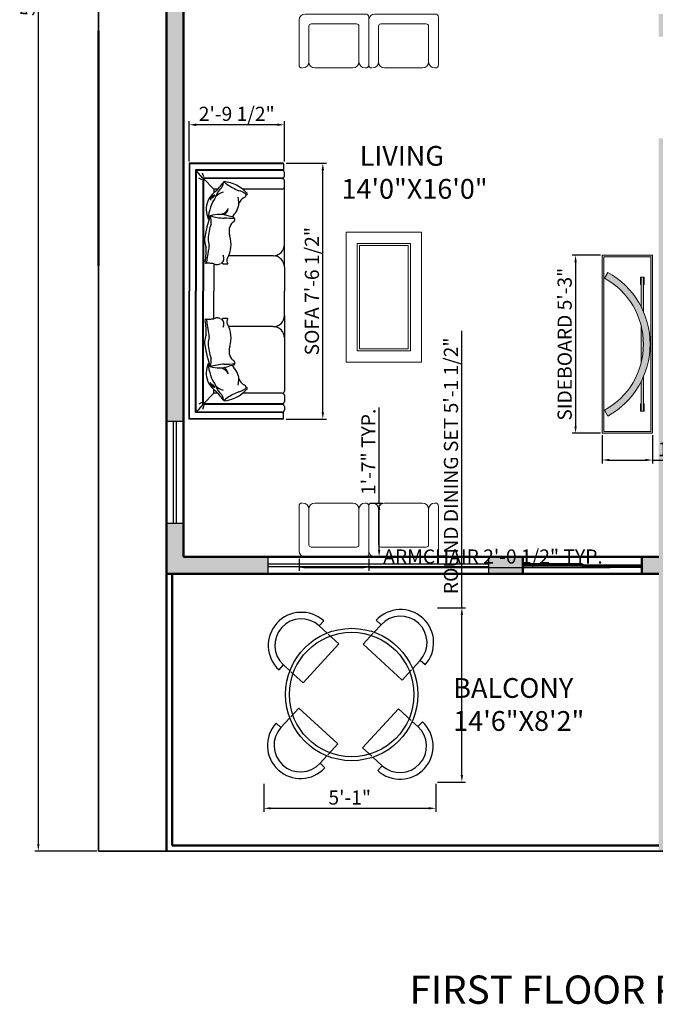
# Model space of a CAD drawing. Units: inches. Extents: x 2638 to 4577, y 1946 to 2619.
# Tile 4 of 8: x 3059 to 3284, y 1946 to 2294. Entities that reach past the tile are written whole.
import ezdxf

# ---------------------------------------------------------------- set-up
doc = ezdxf.new("R2010")
doc.units = ezdxf.units.IN
for name, color, linetype, lineweight in [('A-ANNO-DIMS', 2, 'Continuous', 18), ('A-ANNO-TEXT', 7, 'Continuous', 25), ('A-AREA-IDEN', 7, 'Continuous', 25), ('A-FURN', 8, 'Continuous', 18), ('A-GLAZ', 4, 'Continuous', 25), ('A-WALL', 7, 'Continuous', 50), ('A-WALL-PATT', 8, 'Continuous', 13), ('aparador', 36, 'Continuous', 9), ('C-PROP', 1, 'Continuous', 35), ('moveis', 254, 'Continuous', 5)]:
    doc.layers.add(name, color=color, linetype=linetype, lineweight=lineweight)
doc.layers.add('ESYA', color=11, linetype='Continuous')
doc.layers.add('furn', color=7, linetype='Continuous')
doc.styles.get("Standard").update_dxf_attribs({"font": 'arial.ttf'})
doc.dimstyles.new('ISO-25', dxfattribs={"dimtxt": 5, "dimasz": 2.5, "dimexe": 1.25, "dimexo": 0.625, "dimtad": 1, "dimdec": 1, "dimlunit": 3, "dimtxsty": 'Standard', "dimcen": 2.5, "dimclrt": 1, "dimadec": 0, "dimazin": 0, "dimtfac": 1, "dimtdec": 1, "dimtmove": 0, "dimatfit": 3, "dimfxl": 1, "dimarcsym": 0})

# ---------------------------------------------------------------- blocks, each defined once
blk = doc.blocks.new('*D7')
at = {"layer": 'A-ANNO-DIMS', "color": 0, "lineweight": -2, "transparency": 16777216}
for p, q in [((3086.37, 2600.16), (3064.44, 2600.16)), ((3065.69, 2597.66), (3065.69, 2002.66)), ((3086.37, 2000.16), (3064.44, 2000.16))]:
    blk.add_line(p, q, dxfattribs=at)
at = {"layer": 'A-ANNO-DIMS', "color": 0, "transparency": 16777216}
for points in [[(3065.28, 2597.66), (3066.11, 2597.66), (3065.69, 2600.16)], [(3065.28, 2002.66), (3066.11, 2002.66), (3065.69, 2000.16)]]:
    blk.add_solid(points, dxfattribs=at)
at = {"layer": 'Defpoints', "color": 0, "transparency": 16777216}
for p in [(3086.99, 2600.16), (3065.69, 2000.16), (3086.99, 2000.16)]:
    blk.add_point(p, dxfattribs=at)
at = {"layer": 'A-ANNO-DIMS', "color": 0, "transparency": 16777216, "insert": (3062.52, 2300.16), "char_height": 5, "attachment_point": 5, "rotation": 90}
blk.add_mtext("50'", dxfattribs=at)
blk = doc.blocks.new('Aparador ORGANICA Formatto')
at = {"layer": 'aparador', "ltscale": 0.3}
h = blk.add_hatch(color=256, dxfattribs=at)
h.dxf.hatch_style = 1
h.set_gradient(color1=(118, 213, 123), color2=(52, 168, 57), one_color=1, tint=0.43, name='INVCURVED')
h.paths.add_polyline_path([(0.8, 0.45), (-0.8, 0.45), (-0.8, 0), (0.8, 0)])
h.paths.add_polyline_path([(0.785, 0.435), (0.785, 0.015), (-0.785, 0.015), (-0.785, 0.435)], flags=16)
h.paths.add_polyline_path([(0.2911, 0.3699), (0.5365, 0.3699), (0.5365, 0.3757), (0.6011, 0.3757), (0.6011, 0.3699), (0.6011, 0.3499), (0.6011, 0.3441), (0.5365, 0.3441), (0.5365, 0.3499), (0.3338, 0.3499, -0.150336), (0.6449, 0.0488), (0.5923, 0.0199, 0.208852), (0.1632, 0.3499), (-0.1632, 0.3499, 0.208852), (-0.5923, 0.0199), (-0.6449, 0.0488, -0.150336), (-0.3338, 0.3499), (-0.5365, 0.3499), (-0.5365, 0.3441), (-0.6011, 0.3441), (-0.6011, 0.3499), (-0.6011, 0.3699), (-0.6011, 0.3757), (-0.5365, 0.3757), (-0.5365, 0.3699), (-0.2911, 0.3699, -0.206106)], flags=0)
h = blk.add_hatch(color=256, dxfattribs=at)
h.dxf.hatch_style = 1
h.set_gradient(color1=(135, 92, 69), color2=(0, 0, 0), one_color=1, name='INVCURVED')
h.paths.add_polyline_path([(-0.6449, 0.0488), (-0.5923, 0.0199, -0.590888), (0.5923, 0.0199), (0.6449, 0.0488, 0.590888)])
h = blk.add_hatch(color=256, dxfattribs=at)
h.dxf.hatch_style = 1
h.set_gradient(color1=(178, 189, 189), one_color=1, tint=1, name='CYLINDER')
h.paths.add_polyline_path([(-0.5365, 0.3757), (-0.6011, 0.3757), (-0.6011, 0.3699), (-0.5365, 0.3699)])
h.paths.add_polyline_path([(-0.5365, 0.3499), (-0.6011, 0.3499), (-0.6011, 0.3441), (-0.5365, 0.3441)])
h = blk.add_hatch(color=256, dxfattribs=at)
h.dxf.hatch_style = 1
h.set_gradient(color1=(118, 213, 123), color2=(31, 101, 35), one_color=1, tint=0.26, name='INVCURVED')
h.paths.add_polyline_path([(-0.2911, 0.3699), (-0.6011, 0.3699), (-0.6011, 0.3499), (-0.3338, 0.3499, -0.015999)])
h = blk.add_hatch(color=256, dxfattribs=at)
h.dxf.hatch_style = 1
h.set_gradient(color1=(118, 213, 123), color2=(31, 101, 35), one_color=1, tint=0.26, name='INVCURVED')
h.paths.add_polyline_path([(-0.1632, 0.3499), (0.1632, 0.3499, 0.122516)])
h = blk.add_hatch(color=256, dxfattribs=at)
h.dxf.hatch_style = 1
h.set_gradient(color1=(118, 213, 123), color2=(31, 101, 35), one_color=1, tint=0.26, name='INVCURVED')
h.paths.add_polyline_path([(0.6011, 0.3699), (0.2911, 0.3699, -0.015999), (0.3338, 0.3499), (0.6011, 0.3499)])
h = blk.add_hatch(color=256, dxfattribs=at)
h.dxf.hatch_style = 1
h.set_gradient(color1=(178, 189, 189), one_color=1, tint=1, name='CYLINDER')
h.paths.add_polyline_path([(0.6011, 0.3757), (0.5365, 0.3757), (0.5365, 0.3699), (0.6011, 0.3699)])
h.paths.add_polyline_path([(0.6011, 0.3499), (0.5365, 0.3499), (0.5365, 0.3441), (0.6011, 0.3441)])
for p, q in [((-0.5923, 0.0199), (-0.6449, 0.0488)), ((0.5923, 0.0199), (0.6449, 0.0488))]:
    blk.add_line(p, q, dxfattribs=at)
for points in [[(-0.6011, 0.3699), (-0.6011, 0.3757), (-0.5365, 0.3757), (-0.5365, 0.3699)], [(0.6011, 0.3699), (0.6011, 0.3757), (0.5365, 0.3757), (0.5365, 0.3699)], [(-0.5365, 0.3499), (-0.5365, 0.3441), (-0.6011, 0.3441), (-0.6011, 0.3499)], [(0.5365, 0.3499), (0.5365, 0.3441), (0.6011, 0.3441), (0.6011, 0.3499)]]:
    blk.add_lwpolyline(points, dxfattribs=at)
for radius in [0.7362, 0.6762]:
    blk.add_arc((0, -0.3063), radius, 28.84335, 151.15665, dxfattribs=at)
at = {"layer": 'moveis', "ltscale": 0.3}
for p, q in [((-0.6011, 0.3699), (-0.6011, 0.3499)), ((-0.2911, 0.3699), (-0.6011, 0.3699)), ((0.2911, 0.3699), (0.6011, 0.3699)), ((0.6011, 0.3699), (0.6011, 0.3499)), ((-0.6011, 0.3499), (-0.3338, 0.3499)), ((-0.1632, 0.3499), (0.1632, 0.3499)), ((0.6011, 0.3499), (0.3338, 0.3499))]:
    blk.add_line(p, q, dxfattribs=at)
for points in [[(-0.8, 0), (0.8, 0), (0.8, 0.45), (-0.8, 0.45)], [(-0.785, 0.015), (0.785, 0.015), (0.785, 0.435), (-0.785, 0.435)]]:
    blk.add_lwpolyline(points, close=True, dxfattribs=at)
blk = doc.blocks.new('COUCH6')
at = {"layer": 'furn'}
for p, q in [((-1.1501, -0.8463), (-1.1501, 0)), ((-1.1501, 0), (0, 0)), ((1.1501, 0), (0, 0)), ((1.1501, -0.8463), (1.1501, 0)), ((-1.1451, -0.8463), (-1.1451, -0.005)), ((-1.1451, -0.005), (0, -0.005)), ((-1.0906, -0.8453), (-1.0906, -0.0577)), ((-1.0906, -0.0577), (0, -0.0577)), ((-1.0856, -0.8353), (-1.0856, -0.0627)), ((-1.0856, -0.0627), (0, -0.0627)), ((-1.0164, -0.1236), (-1.0856, -0.0627)), ((-1.0009, -0.1136), (-1.0144, -0.0866)), ((1.1451, -0.005), (0, -0.005)), ((1.0906, -0.0577), (0, -0.0577)), ((1.0856, -0.0627), (0, -0.0627)), ((1.0009, -0.1136), (1.0144, -0.0866)), ((1.0164, -0.1236), (1.0856, -0.0627)), ((1.0856, -0.8353), (1.0856, -0.0627)), ((1.0906, -0.8453), (1.0906, -0.0577)), ((1.1451, -0.8463), (1.1451, -0.005)), ((-1.0263, -0.1311), (-1.0612, -0.1208)), ((-1.0164, -0.8353), (-1.0164, -0.1236)), ((-1.0164, -0.1236), (0, -0.1236)), ((-1.0114, -0.8353), (-1.0114, -0.1286)), ((-1.0114, -0.1286), (0, -0.1286)), ((-0.917, -0.2229), (-1.0114, -0.1286)), ((-0.6507, -0.1709), (-0.6516, -0.1803)), ((1.0164, -0.1236), (0, -0.1236)), ((1.0114, -0.1286), (0, -0.1286)), ((0.6507, -0.1709), (0.6516, -0.1803)), ((0.917, -0.2229), (1.0114, -0.1286)), ((1.0114, -0.8353), (1.0114, -0.1286)), ((1.0164, -0.8353), (1.0164, -0.1236)), ((1.0263, -0.1311), (1.0612, -0.1208)), ((-0.917, -0.2229), (-0.8844, -0.2229)), ((-0.917, -0.259), (-0.917, -0.2229)), ((-0.2469, -0.2229), (0, -0.2229)), ((0.2469, -0.2229), (0, -0.2229)), ((0.917, -0.2229), (0.8844, -0.2229)), ((0.917, -0.259), (0.917, -0.2229)), ((-0.318, -0.7552), (-0.318, -0.3506)), ((-0.665, -0.398), (-0.6739, -0.3593)), ((-0.6508, -0.4092), (-0.665, -0.398)), ((0.318, -0.7552), (0.318, -0.3554)), ((0.6508, -0.4092), (0.665, -0.398)), ((0.665, -0.398), (0.6739, -0.3593)), ((-0.917, -0.8353), (-0.917, -0.48)), ((0.917, -0.8353), (0.917, -0.48)), ((-1.1451, -0.8463), (-1.0916, -0.8463)), ((-1.0906, -0.8353), (-1.0906, -0.8453)), ((-1.0906, -0.8353), (-1.0856, -0.8353)), ((-1.0364, -0.8553), (-1.0656, -0.8553)), ((-0.937, -0.8553), (-0.9914, -0.8553)), ((-0.4181, -0.8553), (-0.897, -0.8553)), ((-0.2179, -0.8553), (-0.4181, -0.8553)), ((-0.2179, -0.8553), (0, -0.8553)), ((0.2179, -0.8553), (0, -0.8553)), ((0.2179, -0.8553), (0.4181, -0.8553)), ((0.4181, -0.8553), (0.9914, -0.8553)), ((0.937, -0.8553), (0.9914, -0.8553)), ((0.937, -0.8553), (0.9914, -0.8553)), ((1.0364, -0.8553), (1.0656, -0.8553)), ((1.0906, -0.8353), (1.0856, -0.8353)), ((1.0906, -0.8353), (1.0906, -0.8453)), ((1.1451, -0.8463), (1.0916, -0.8463))]:
    blk.add_line(p, q, dxfattribs=at)
for centre, radius, start, end in [((-0.6935, -0.4002), 0.2605, 116.61716, 144.57015), ((-0.6199, -0.5798), 0.41, 94.3064, 124.24766), ((-0.7351, -0.3719), 0.218, 67.21953, 110.1562), ((-0.3903, -0.9655), 0.8275, 98.67557, 110.29795), ((-0.4352, -0.6995), 0.5297, 93.94951, 108.49156), ((-0.4612, -0.298), 0.16, 64.49689, 109.71288), ((-0.4636, -0.3121), 0.1412, 68.12041, 93.31004), ((-0.4019, -0.0788), 0.1026, 264.95348, 292.56183), ((-0.3738, 0.4077), 0.5616, 268.1099, 280.95976), ((-0.4941, 1.0065), 1.1874, 276.3584, 281.81637), ((-0.2605, -0.1517), 0.0104, 337.65411, 129.2107), ((0.3523, -0.1787), 0.6036, 177.81706, 180.67732), ((0.2605, -0.1517), 0.0104, 50.7893, 202.34589), ((-0.3523, -0.1787), 0.6036, 359.32268, 2.18294), ((0.4941, 1.0065), 1.1874, 258.18363, 263.6416), ((0.3738, 0.4077), 0.5616, 259.04024, 271.8901), ((0.4019, -0.0788), 0.1026, 247.43817, 275.04652), ((0.4612, -0.298), 0.16, 70.28712, 115.50311), ((0.4636, -0.3121), 0.1412, 86.68996, 111.87959), ((0.4352, -0.6995), 0.5297, 71.50844, 86.05049), ((0.3903, -0.9655), 0.8275, 69.70205, 81.32443), ((0.7351, -0.3719), 0.218, 69.8438, 112.78047), ((0.6199, -0.5798), 0.41, 55.75234, 85.6936), ((0.6935, -0.4002), 0.2605, 35.42985, 63.38284), ((-1.737, 0.6879), 1.2526, 306.90338, 311.57577), ((-0.8085, -0.3921), 0.157, 105.54086, 140.99269), ((-0.7757, -0.3273), 0.1143, 130.90927, 169.83826), ((-0.8227, -0.2301), 0.0392, 84.92852, 182.67064), ((-0.8092, -0.2372), 0.0473, 102.3256, 174.63718), ((-0.8175, -0.2488), 0.0419, 116.14342, 157.62806), ((-0.4135, -0.2689), 0.2757, 163.22567, 199.12388), ((-1.2327, -0.3515), 0.5785, 3.57396, 16.27286), ((-0.6254, -0.0511), 0.1477, 249.39872, 278.63857), ((0.4923, -0.1174), 0.7467, 185.25446, 188.12337), ((-0.3322, -0.2403), 0.0937, 332.69161, 351.86349), ((-0.3066, -0.2538), 0.0672, 0.19522, 27.37766), ((0.3066, -0.2538), 0.0672, 152.62234, 179.80478), ((0.3322, -0.2403), 0.0937, 188.13651, 207.30839), ((-0.4923, -0.1174), 0.7467, 351.87663, 354.74554), ((0.6254, -0.0511), 0.1477, 261.36143, 290.60128), ((1.2327, -0.3515), 0.5785, 163.72714, 176.42604), ((0.4135, -0.2689), 0.2757, 340.87612, 16.77433), ((0.8227, -0.2301), 0.0392, 357.32936, 95.07148), ((0.8092, -0.2372), 0.0473, 5.36282, 77.6744), ((0.8175, -0.2488), 0.0419, 22.37194, 63.85658), ((0.7757, -0.3273), 0.1143, 10.16174, 49.09073), ((0.8085, -0.3921), 0.157, 39.00731, 74.45914), ((1.737, 0.6879), 1.2526, 228.42423, 233.09662), ((-1.1356, 0.1688), 0.5056, 287.35579, 293.93444), ((-1.0472, -0.3998), 0.1063, 32.17608, 54.05242), ((-0.6626, -0.2793), 0.3241, 186.10693, 226.96204), ((-1.5696, -0.7286), 0.7236, 22.89192, 32.18565), ((-0.7783, -0.2698), 0.0893, 293.17936, 356.91871), ((-0.7589, -0.2677), 0.0857, 280.6079, 328.64782), ((0.513, -0.3052), 1.1684, 180.49863, 185.10663), ((-0.4205, -0.1158), 0.2606, 252.95174, 298.53043), ((-0.296, -0.2474), 0.0649, 245.50719, 314.42583), ((-0.2725, -0.3894), 0.0505, 58.55463, 117.80385), ((-0.2311, -0.2915), 0.0196, 155.48458, 217.91726), ((-0.4058, -0.3264), 0.1609, 352.88429, 8.17531), ((0.4058, -0.3264), 0.1609, 171.82469, 187.11571), ((0.2725, -0.3894), 0.0505, 62.19615, 121.44537), ((0.2311, -0.2915), 0.0196, 322.08274, 24.51542), ((0.296, -0.2474), 0.0649, 225.57417, 294.49281), ((0.4205, -0.1158), 0.2606, 241.46957, 287.04826), ((-0.513, -0.3052), 1.1684, 354.89337, 359.50137), ((0.7589, -0.2677), 0.0857, 211.35218, 259.3921), ((0.7783, -0.2698), 0.0893, 183.08129, 246.82064), ((0.6626, -0.2793), 0.3241, 313.03796, 353.89307), ((1.5696, -0.7286), 0.7236, 147.81435, 157.10808), ((1.1356, 0.1688), 0.5056, 246.06556, 252.64421), ((1.0472, -0.3998), 0.1063, 125.94758, 147.82392), ((-0.767, -0.1224), 0.3263, 256.45311, 265.96892), ((-0.8131, -0.2526), 0.1966, 276.76881, 317.60176), ((-0.6432, -0.3863), 0.0242, 251.75441, 345.55562), ((-0.5365, -0.4767), 0.1185, 70.4821, 134.60789), ((0.5365, -0.4767), 0.1185, 45.39211, 109.5179), ((0.6432, -0.3863), 0.0242, 194.44438, 288.24559), ((0.8131, -0.2526), 0.1966, 222.39824, 263.23119), ((0.767, -0.1224), 0.3263, 274.03108, 283.54689), ((-0.7549, -0.4097), 0.1528, 194.18022, 223.19602), ((-0.8752, -0.514), 0.00886, 194.0721, 357.96189), ((-0.876, -0.4776), 0.038, 284.83159, 343.52549), ((-0.7217, -0.5822), 0.1507, 116.94283, 141.47936), ((0.7217, -0.5822), 0.1507, 38.52064, 63.05717), ((0.876, -0.4776), 0.038, 196.47451, 255.16841), ((0.7549, -0.4097), 0.1528, 316.80398, 345.81978), ((0.8752, -0.514), 0.00886, 182.03811, 345.9279), ((-0.4181, -0.7552), 0.1001, 270, 0), ((-0.2179, -0.7552), 0.1001, 180, 270), ((0.2179, -0.7552), 0.1001, 270, 0), ((0.4181, -0.7552), 0.1001, 180, 270), ((-1.1476, -0.8463), 0.0025, 180, 0), ((-1.0916, -0.8453), 0.001, 270, 0), ((-1.0916, -0.8453), 0.001, 270, 0), ((-1.0916, -0.8453), 0.001, 270, 0), ((-1.0656, -0.8353), 0.02, 180, 270), ((-1.0364, -0.8353), 0.02, 270, 0), ((-1.0139, -0.8353), 0.0025, 180, 0), ((-0.9914, -0.8353), 0.02, 180, 270), ((-0.937, -0.8353), 0.02, 270, 360), ((-0.897, -0.8353), 0.02, 180, 270), ((0.937, -0.8353), 0.02, 180, 270), ((0.9914, -0.8353), 0.02, 270, 0), ((1.0139, -0.8353), 0.0025, 180, 0), ((1.0364, -0.8353), 0.02, 180, 270), ((1.0656, -0.8353), 0.02, 270, 0), ((1.0916, -0.8453), 0.001, 180, 270), ((1.0916, -0.8453), 0.001, 180, 270), ((1.0916, -0.8453), 0.001, 180, 270), ((1.1476, -0.8463), 0.0025, 180, 0)]:
    blk.add_arc(centre, radius, start, end, dxfattribs=at)
blk = doc.blocks.new('sofa-27')
at = {"color": 0, "linetype": 'ByBlock'}
for p, q in [((-0.0591, 0.0591), (-0.0591, 0.4902)), ((0.0945, 0.5198), (0.459, 0.5198)), ((0.6125, 0.0295), (0.6125, 0.4902)), ((0.0354, 0.1181), (0.0354, 0.4607)), ((0.518, 0.1181), (0.518, 0.4607)), ((0.583, 0), (0, 0)), ((0.4944, 0.0945), (0.0591, 0.0945))]:
    blk.add_line(p, q, dxfattribs=at)
for centre, radius, start, end in [((-0.0295, 0.4902), 0.0295, 90, 180), ((-0.0236, 0.4607), 0.0591, 360, 90), ((0.0945, 0.4607), 0.0591, 90, 180), ((0.459, 0.4607), 0.0591, 0, 90), ((0.5771, 0.4607), 0.0591, 90, 180), ((0.583, 0.4902), 0.0295, 0, 90), ((0.0591, 0.1181), 0.0236, 180, 270), ((0.4944, 0.1181), 0.0236, 270, 0), ((0, 0.0591), 0.0591, 180, 270), ((0.583, 0.0295), 0.0295, 270, 0)]:
    blk.add_arc(centre, radius, start, end, dxfattribs=at)
blk = doc.blocks.new('HBBJVBGFGJG')
at = {"layer": 'ESYA'}
for p, q in [((60816.41, -8226.23), (60813.04, -8229.93)), ((60856.02, -8225.76), (60859.71, -8229.13)), ((60813.04, -8229.93), (60819.01, -8235.38)), ((60859.71, -8229.13), (60854.55, -8234.79)), ((60819.83, -8236.13), (60827.81, -8243.41)), ((60853.82, -8235.59), (60846.23, -8243.9)), ((60827.81, -8243.41), (60800.84, -8272.95)), ((60846.23, -8243.9), (60875.77, -8270.87)), ((60883.59, -8262.31), (60889.25, -8256.1)), ((60892.94, -8259.48), (60889.25, -8256.1)), ((60782.69, -8263.16), (60786.07, -8259.46)), ((60790.88, -8263.86), (60786.07, -8259.46)), ((60800.84, -8272.95), (60791.67, -8264.59)), ((60875.77, -8270.87), (60882.84, -8263.12)), ((60791.53, -8298.66), (60797.61, -8292.01)), ((60797.61, -8292.01), (60827.14, -8318.98)), ((60845.82, -8322.1), (60872.79, -8292.56)), ((60872.79, -8292.56), (60882.46, -8301.4)), ((60784.12, -8306.78), (60790.78, -8299.49)), ((60883.24, -8302.11), (60887.56, -8306.05)), ((60890.93, -8302.36), (60887.56, -8306.05)), ((60780.43, -8303.41), (60784.12, -8306.78)), ((60827.14, -8318.98), (60819.49, -8327.36)), ((60852.72, -8328.4), (60845.82, -8322.1)), ((60818.77, -8328.15), (60813.66, -8333.75)), ((60860.58, -8335.59), (60853.57, -8329.18)), ((60817.35, -8337.12), (60813.66, -8333.75)), ((60857.21, -8339.28), (60860.58, -8335.59))]:
    blk.add_line(p, q, dxfattribs=at)
for radius in [50, 47]:
    blk.add_circle((60837.55, -8281.81), radius, dxfattribs=at)
for centre, radius, start, end in [((60799.55, -8244.7), 25, 47.59911, 227.59911), ((60874.48, -8242.62), 25, 317.59911, 137.59911), ((60799.55, -8244.7), 20, 47.59911, 227.59911), ((60874.48, -8242.62), 20, 317.59911, 137.59911), ((60874.07, -8320.82), 25, 227.59911, 47.59911), ((60798.89, -8320.27), 25, 137.59911, 317.59911), ((60798.89, -8320.27), 20, 137.59911, 317.59911), ((60874.07, -8320.82), 20, 227.59911, 47.59911)]:
    blk.add_arc(centre, radius, start, end, dxfattribs=at)
blk = doc.blocks.new('WIN-36')
for p, q in [((2761.41, 2540.16), (2761.41, 2534.16)), ((2797.41, 2540.16), (2797.41, 2534.16)), ((2761.41, 2537.66), (2797.41, 2537.66)), ((2761.41, 2536.66), (2797.41, 2536.66))]:
    blk.add_line(p, q)
blk = doc.blocks.new('WIN-78')
for p, q in [((3314.99, 2024.16), (3314.99, 2018.16)), ((3392.99, 2024.16), (3392.99, 2018.16)), ((3314.99, 2021.66), (3392.99, 2021.66)), ((3314.99, 2020.66), (3392.99, 2020.66))]:
    blk.add_line(p, q)
blk = doc.blocks.new('*D55')
at = {"layer": 'A-ANNO-DIMS', "color": 0, "lineweight": -2, "transparency": 16777216}
for p, q in [((3157.84, 2103.53), (3157.84, 2099.21)), ((3182.46, 2103.53), (3182.46, 2099.21)), ((3160.34, 2100.46), (3179.96, 2100.46)), ((3182.46, 2100.46), (3267.83, 2100.46))]:
    blk.add_line(p, q, dxfattribs=at)
at = {"layer": 'A-ANNO-DIMS', "color": 0, "transparency": 16777216}
for points in [[(3160.34, 2100.88), (3160.34, 2100.05), (3157.84, 2100.46)], [(3179.96, 2100.88), (3179.96, 2100.05), (3182.46, 2100.46)]]:
    blk.add_solid(points, dxfattribs=at)
at = {"layer": 'Defpoints', "color": 0, "transparency": 16777216}
for p in [(3157.84, 2104.16), (3182.46, 2104.16), (3182.46, 2100.46)]:
    blk.add_point(p, dxfattribs=at)
at = {"layer": 'A-ANNO-DIMS', "color": 1, "transparency": 16777216, "insert": (3226.4, 2103.67), "char_height": 5, "attachment_point": 5}
blk.add_mtext('ARMCHAIR 2\'-0 1/2" TYP.', dxfattribs=at)
blk = doc.blocks.new('*D56')
at = {"layer": 'A-ANNO-DIMS', "color": 0, "lineweight": -2, "transparency": 16777216}
for p, q in [((3186.16, 2123.21), (3186.16, 2156.97)), ((3183.09, 2123.21), (3187.41, 2123.21)), ((3186.16, 2106.66), (3186.16, 2120.71)), ((3183.09, 2104.16), (3187.41, 2104.16))]:
    blk.add_line(p, q, dxfattribs=at)
at = {"layer": 'A-ANNO-DIMS', "color": 0, "transparency": 16777216}
for points in [[(3185.74, 2120.71), (3186.57, 2120.71), (3186.16, 2123.21)], [(3185.74, 2106.66), (3186.57, 2106.66), (3186.16, 2104.16)]]:
    blk.add_solid(points, dxfattribs=at)
at = {"layer": 'Defpoints', "color": 0, "transparency": 16777216}
for p in [(3182.46, 2123.21), (3186.16, 2123.21), (3182.46, 2104.16)]:
    blk.add_point(p, dxfattribs=at)
at = {"layer": 'A-ANNO-DIMS', "color": 1, "transparency": 16777216, "insert": (3183.02, 2141.34), "char_height": 5, "attachment_point": 5, "rotation": 90}
blk.add_mtext('1\'-7" TYP.', dxfattribs=at)
blk = doc.blocks.new('*D75')
at = {"layer": 'A-ANNO-DIMS', "color": 0, "lineweight": -2, "transparency": 16777216}
for p, q in [((3264.42, 2210.88), (3254.34, 2210.88)), ((3255.59, 2208.38), (3255.59, 2150.39)), ((3264.42, 2147.89), (3254.34, 2147.89))]:
    blk.add_line(p, q, dxfattribs=at)
at = {"layer": 'A-ANNO-DIMS', "color": 0, "transparency": 16777216}
for points in [[(3255.18, 2208.38), (3256.01, 2208.38), (3255.59, 2210.88)], [(3255.18, 2150.39), (3256.01, 2150.39), (3255.59, 2147.89)]]:
    blk.add_solid(points, dxfattribs=at)
at = {"layer": 'Defpoints', "color": 0, "transparency": 16777216}
for p in [(3265.04, 2210.88), (3255.59, 2147.89), (3265.04, 2147.89)]:
    blk.add_point(p, dxfattribs=at)
at = {"layer": 'A-ANNO-DIMS', "color": 1, "transparency": 16777216, "insert": (3252.38, 2179.39), "char_height": 5, "attachment_point": 5, "rotation": 90}
blk.add_mtext('SIDEBOARD 5\'-3"', dxfattribs=at)
blk = doc.blocks.new('*D76')
at = {"layer": 'A-ANNO-DIMS', "color": 0, "lineweight": -2, "transparency": 16777216}
for p, q in [((3265.04, 2147.27), (3265.04, 2137.19)), ((3282.76, 2147.27), (3282.76, 2137.19)), ((3267.54, 2138.44), (3280.26, 2138.44)), ((3282.76, 2138.44), (3310.98, 2138.44))]:
    blk.add_line(p, q, dxfattribs=at)
at = {"layer": 'A-ANNO-DIMS', "color": 0, "transparency": 16777216}
for points in [[(3267.54, 2138.86), (3267.54, 2138.03), (3265.04, 2138.44)], [(3280.26, 2138.86), (3280.26, 2138.03), (3282.76, 2138.44)]]:
    blk.add_solid(points, dxfattribs=at)
at = {"layer": 'Defpoints', "color": 0, "transparency": 16777216}
for p in [(3265.04, 2147.89), (3282.76, 2147.89), (3282.76, 2138.44)]:
    blk.add_point(p, dxfattribs=at)
at = {"layer": 'A-ANNO-DIMS', "color": 1, "transparency": 16777216, "insert": (3298.12, 2141.65), "char_height": 5, "attachment_point": 5}
blk.add_mtext('1\'-5 1/2"', dxfattribs=at)
blk = doc.blocks.new('*D89')
at = {"layer": 'A-ANNO-DIMS', "color": 0, "lineweight": -2, "transparency": 16777216}
for p, q in [((3153.29, 2243.42), (3167.5, 2243.42)), ((3166.25, 2155.36), (3166.25, 2240.92)), ((3153.29, 2152.86), (3167.5, 2152.86))]:
    blk.add_line(p, q, dxfattribs=at)
at = {"layer": 'A-ANNO-DIMS', "color": 0, "transparency": 16777216}
for points in [[(3165.83, 2240.92), (3166.67, 2240.92), (3166.25, 2243.42)], [(3165.83, 2155.36), (3166.67, 2155.36), (3166.25, 2152.86)]]:
    blk.add_solid(points, dxfattribs=at)
at = {"layer": 'Defpoints', "color": 0, "transparency": 16777216}
for p in [(3152.67, 2243.42), (3166.25, 2243.42), (3152.67, 2152.86)]:
    blk.add_point(p, dxfattribs=at)
at = {"layer": 'A-ANNO-DIMS', "color": 1, "transparency": 16777216, "insert": (3163.04, 2198.14), "char_height": 5, "attachment_point": 5, "rotation": 90}
blk.add_mtext('SOFA 7\'-6 1/2"', dxfattribs=at)
blk = doc.blocks.new('*D90')
at = {"layer": 'A-ANNO-DIMS', "color": 0, "lineweight": -2, "transparency": 16777216}
for p, q in [((3118.99, 2244.04), (3118.99, 2258.25)), ((3150.17, 2257), (3121.49, 2257)), ((3152.67, 2244.04), (3152.67, 2258.25))]:
    blk.add_line(p, q, dxfattribs=at)
at = {"layer": 'A-ANNO-DIMS', "color": 0, "transparency": 16777216}
for points in [[(3121.49, 2257.42), (3121.49, 2256.58), (3118.99, 2257)], [(3150.17, 2257.42), (3150.17, 2256.58), (3152.67, 2257)]]:
    blk.add_solid(points, dxfattribs=at)
at = {"layer": 'Defpoints', "color": 0, "transparency": 16777216}
for p in [(3118.99, 2257), (3118.99, 2243.42), (3152.67, 2243.42)]:
    blk.add_point(p, dxfattribs=at)
at = {"layer": 'A-ANNO-DIMS', "color": 1, "transparency": 16777216, "insert": (3135.83, 2260.21), "char_height": 5, "attachment_point": 5}
blk.add_mtext('2\'-9 1/2"', dxfattribs=at)
blk = doc.blocks.new('*D91')
at = {"layer": 'A-ANNO-DIMS', "color": 0, "lineweight": -2, "transparency": 16777216}
for p, q in [((3215.41, 2086.19), (3215.41, 2184.09)), ((3206.78, 2086.19), (3216.66, 2086.19)), ((3215.41, 2027.03), (3215.41, 2083.69)), ((3206.78, 2024.53), (3216.66, 2024.53))]:
    blk.add_line(p, q, dxfattribs=at)
at = {"layer": 'A-ANNO-DIMS', "color": 0, "transparency": 16777216}
for points in [[(3214.99, 2083.69), (3215.82, 2083.69), (3215.41, 2086.19)], [(3214.99, 2027.03), (3215.82, 2027.03), (3215.41, 2024.53)]]:
    blk.add_solid(points, dxfattribs=at)
at = {"layer": 'Defpoints', "color": 0, "transparency": 16777216}
for p in [(3206.16, 2086.19), (3215.41, 2086.19), (3206.16, 2024.53)]:
    blk.add_point(p, dxfattribs=at)
at = {"layer": 'A-ANNO-DIMS', "color": 1, "transparency": 16777216, "insert": (3212.19, 2136.39), "char_height": 5, "attachment_point": 5, "rotation": 90}
blk.add_mtext('ROUND DINING SET 5\'-1 1/2"', dxfattribs=at)
blk = doc.blocks.new('*D92')
at = {"layer": 'A-ANNO-DIMS', "color": 0, "lineweight": -2, "transparency": 16777216}
for p, q in [((3145.36, 2023.9), (3145.36, 2014.03)), ((3206.16, 2023.9), (3206.16, 2014.03)), ((3147.86, 2015.28), (3203.66, 2015.28))]:
    blk.add_line(p, q, dxfattribs=at)
at = {"layer": 'A-ANNO-DIMS', "color": 0, "transparency": 16777216}
for points in [[(3147.86, 2015.69), (3147.86, 2014.86), (3145.36, 2015.28)], [(3203.66, 2015.69), (3203.66, 2014.86), (3206.16, 2015.28)]]:
    blk.add_solid(points, dxfattribs=at)
at = {"layer": 'Defpoints', "color": 0, "transparency": 16777216}
for p in [(3145.36, 2024.53), (3206.16, 2024.53), (3206.16, 2015.28)]:
    blk.add_point(p, dxfattribs=at)
at = {"layer": 'A-ANNO-DIMS', "color": 1, "transparency": 16777216, "insert": (3175.76, 2018.45), "char_height": 5, "attachment_point": 5}
blk.add_mtext('5\'-1"', dxfattribs=at)

msp = doc.modelspace()

# ---------------------------------------------------------------- hatches: boundary and pattern name
at = {"layer": 'A-WALL-PATT', "transparency": 33554687}
h = msp.add_hatch(color=256, dxfattribs=at)
h.dxf.hatch_style = 1
h.paths.add_polyline_path([(3116.99, 2552.16), (3137.99, 2552.16), (3137.99, 2558.16), (3110.99, 2558.16), (3110.99, 2507.16), (3116.99, 2507.16)])
h.paths.add_polyline_path([(3252.94, 2558.16), (3179.99, 2558.16), (3179.99, 2552.16), (3194.4, 2552.16), (3252.94, 2552.16)])
h.paths.add_polyline_path([(3422.99, 2558.16), (3288.94, 2558.16), (3288.94, 2552.16), (3318.99, 2552.16), (3318.99, 2532.16), (3322.99, 2532.16), (3322.99, 2552.16), (3416.99, 2552.16), (3416.99, 2492.16), (3354.99, 2492.16), (3354.99, 2488.16), (3416.99, 2488.16), (3416.99, 2481.16), (3422.99, 2481.16)])
h.paths.add_polyline_path([(3422.99, 2457.16), (3416.99, 2457.16), (3416.99, 2426.16), (3372.26, 2426.16), (3322.99, 2426.16), (3322.99, 2439.06), (3322.99, 2488.16), (3324.99, 2488.16), (3324.99, 2492.16), (3322.99, 2492.16), (3322.99, 2502.16), (3318.99, 2502.16), (3318.99, 2426.16), (3297.01, 2426.16), (3296.99, 2422.16), (3416.99, 2422.16), (3416.99, 2418.91), (3422.99, 2418.91)])
h.paths.add_polyline_path([(3146.99, 2104.16), (3116.99, 2104.16), (3116.99, 2116.16), (3110.99, 2116.16), (3110.99, 2098.16), (3146.99, 2098.16)])
h.paths.add_polyline_path([(3236.99, 2104.16), (3224.99, 2104.16), (3224.99, 2098.16), (3236.99, 2098.16)])
h.paths.add_polyline_path([(3290.99, 2252.16), (3284.99, 2252.16), (3284.99, 2104.16), (3278.99, 2104.16), (3278.99, 2098.16), (3284.99, 2098.16), (3284.99, 2000.16), (3290.99, 2000.16), (3290.99, 2018.16), (3314.99, 2018.16), (3314.99, 2024.16), (3290.99, 2024.16)])
h.paths.add_polyline_path([(3422.99, 2060.16), (3416.99, 2060.16), (3416.99, 2024.16), (3392.99, 2024.16), (3392.99, 2018.16), (3422.99, 2018.16)])
h.paths.add_polyline_path([(3422.99, 2244.16), (3416.99, 2244.16), (3416.99, 2220.16), (3372.26, 2220.16), (3338.99, 2220.16), (3338.99, 2222.16), (3334.99, 2222.16), (3334.99, 2216.16), (3416.99, 2216.16), (3416.99, 2096.16), (3422.99, 2096.16)])
h.paths.add_polyline_path([(3422.99, 2300.41), (3416.99, 2300.41), (3416.99, 2296.16), (3284.99, 2296.16), (3284.99, 2288.16), (3290.99, 2288.16), (3290.99, 2292.16), (3334.99, 2292.16), (3334.99, 2252.16), (3338.99, 2252.16), (3338.99, 2292.16), (3416.99, 2292.16), (3416.99, 2268.16), (3422.99, 2268.16)])
h.paths.add_polyline_path([(3422.99, 2382.91), (3416.99, 2382.91), (3416.99, 2336.41), (3422.99, 2336.41)])
h.paths.add_polyline_path([(3260.99, 2426.16), (3116.99, 2426.16), (3116.99, 2471.16), (3110.99, 2471.16), (3110.99, 2404.16), (3116.99, 2404.16), (3116.99, 2422.16), (3260.99, 2422.16)])
h.paths.add_polyline_path([(3116.99, 2320.16), (3110.99, 2320.16), (3110.99, 2152.16), (3116.99, 2152.16)])
h.paths.add_polyline_path([(3192.92, 2481.2), (3252.23, 2481.2), (3252.23, 2507.82), (3192.92, 2507.82)], flags=9)
h.paths.add_polyline_path([(3352.38, 2202.6), (3398.15, 2202.6), (3398.15, 2210.84), (3352.38, 2210.84)], flags=25)
h.paths.add_polyline_path([(3108.13, 2334.43), (3108.13, 2401.53), (3093.19, 2401.53), (3093.19, 2334.43)], flags=9)
h.paths.add_polyline_path([(3441.94, 2334.43), (3441.94, 2401.53), (3426.99, 2401.53), (3426.99, 2334.43)], flags=9)
h.paths.add_polyline_path([(3282.12, 2570.46), (3349.22, 2570.46), (3349.22, 2585.4), (3282.12, 2585.4)], flags=9)
h.paths.add_polyline_path([(3240.15, 2347.41), (3289.11, 2347.41), (3289.11, 2374.03), (3240.15, 2374.03)], flags=9)
h.paths.add_polyline_path([(3169.91, 2226.85), (3224.05, 2226.85), (3224.05, 2253.46), (3169.91, 2253.46)], flags=9)
h.paths.add_polyline_path([(3209.4, 2038.68), (3263.9, 2038.68), (3263.9, 2065.29), (3209.4, 2065.29)], flags=9)
h.paths.add_polyline_path([(3313.05, 2123.44), (3369.27, 2123.44), (3369.27, 2150.05), (3313.05, 2150.05)], flags=9)
h.paths.add_polyline_path([(3359.46, 2259.32), (3395.23, 2259.32), (3395.23, 2278.33), (3359.46, 2278.33)], flags=25)

# ---------------------------------------------------------------- linework, layer by layer
at = {"layer": 'A-FURN'}
for points in [[(3174.45, 2173.07), (3201.14, 2173.07), (3201.14, 2218.98), (3174.45, 2218.98)], [(3178.38, 2177.01), (3197.2, 2177.01), (3197.2, 2215.04), (3178.38, 2215.04)], [(3179.17, 2177.8), (3196.41, 2177.8), (3196.41, 2214.25), (3179.17, 2214.25)]]:
    msp.add_lwpolyline(points, close=True, dxfattribs=at)
at = {"layer": 'A-WALL'}
for p, q in [((3110.99, 2000.16), (3110.99, 2594.16)), ((3116.99, 2104.16), (3116.99, 2422.16)), ((3086.99, 2207.16), (3086.99, 2290.16)), ((3284.99, 2104.16), (3116.99, 2104.16)), ((3236.99, 2104.16), (3236.99, 2098.16)), ((3278.99, 2104.16), (3278.99, 2098.16)), ((3236.99, 2101.66), (3257.99, 2101.66)), ((3236.99, 2101.16), (3278.99, 2101.16)), ((3257.99, 2101.66), (3257.99, 2100.66)), ((3257.99, 2100.66), (3278.99, 2100.66)), ((3284.99, 2098.16), (3110.99, 2098.16)), ((3112.99, 2002.16), (3112.99, 2098.16)), ((3284.99, 2002.16), (3112.99, 2002.16))]:
    msp.add_line(p, q, dxfattribs=at)
at = {"layer": 'C-PROP'}
msp.add_lwpolyline([(3086.99, 2600.16), (3446.99, 2600.16), (3446.99, 2000.16), (3086.99, 2000.16)], close=True, dxfattribs=at)

# ---------------------------------------------------------------- block references
at = {"layer": 'A-FURN'}
for name, p, xscale, yscale, zscale, rotation in [('sofa-27', (3160.01, 2296.16), -36.66436083614781, 36.66436083614781, 36.66436083614781, 180), ('sofa-27', (3184.63, 2296.16), -36.66436083614781, 36.66436083614781, 36.66436083614781, 180), ('COUCH6', (3118.99, 2198.14), 39.3701, 39.3701, 39.3701, 90.00000000000003), ('Aparador ORGANICA Formatto', (3265.04, 2179.39), 39.3701, 39.3701, 39.3701, 270)]:
    msp.add_blockref(name, p, dxfattribs=dict(at, xscale=xscale, yscale=yscale, zscale=zscale, rotation=rotation))
for name, p, xscale, yscale, zscale in [('sofa-27', (3160.01, 2104.16), 36.66436083614781, 36.66436083614781, 36.66436083614781), ('sofa-27', (3184.63, 2104.16), 36.66436083614781, 36.66436083614781, 36.66436083614781), ('HBBJVBGFGJG', (-25297.37, 5931.66), 0.4680303905490205, 0.4680303905490205, 0.4680303905490205)]:
    msp.add_blockref(name, p, dxfattribs=dict(at, xscale=xscale, yscale=yscale, zscale=zscale))
at = {"layer": 'A-GLAZ'}
for name, p, rotation in [('WIN-36', (5651.15, -645.25), 90.00000000000443), ('WIN-78', (6539.98, 4122.31), 180)]:
    msp.add_blockref(name, p, dxfattribs=dict(at, rotation=rotation))

# ---------------------------------------------------------------- texts
at = {"layer": 'A-ANNO-TEXT', "insert": (3196.91, 1956.14), "char_height": 10, "attachment_point": 1}
msp.add_mtext_dynamic_manual_height_columns('{\\fTimes New Roman|b0|i0|c0|p18;FIRST FLOOR PLAN}', width=196.2607, gutter_width=12.5, heights=[0], dxfattribs=at)
at = {"layer": 'A-AREA-IDEN', "char_height": 7, "attachment_point": 1}
for s, insert in [('{\\fTimes New Roman|b0|i0|c0|p18;   LIVING\\P14\'0"X16\'0"}', (3172.87, 2249.5)), ('{\\fTimes New Roman|b0|i0|c0|p18;BALCONY\\P14\'6"X8\'2"}', (3212.36, 2061.33))]:
    msp.add_mtext_dynamic_manual_height_columns(s, width=61.0557, gutter_width=12.5, heights=[0], dxfattribs=dict(at, insert=insert))

# ---------------------------------------------------------------- dimensions: what is measured, and where the dimension line sits
at = {"layer": 'A-ANNO-DIMS'}
for base, p1, p2, angle, override, picture, middle in [((3065.69, 2000.16), (3086.99, 2600.16), (3086.99, 2000.16), 90, {"dimclrd": 0, "dimclre": 0, "dimclrt": 0}, '*D7', (3062.52, 2300.16)), ((3118.99, 2257), (3152.67, 2243.42), (3118.99, 2243.42), 180, {"dimdec": 1, "dimrnd": 0, "dimzin": 1, "dimlunit": 4, "dimfrac": 2}, '*D90', (3135.83, 2260.21))]:
    dim = msp.add_linear_dim(base=base, p1=p1, p2=p2, angle=angle, dimstyle='ISO-25', override=override, dxfattribs=at)
    dim.commit()
    dim.dimension.update_dxf_attribs({"geometry": picture, "text_midpoint": middle})
for base, p1, p2, angle, text, picture, middle in [((3166.25, 2243.42), (3152.67, 2152.86), (3152.67, 2243.42), 90, 'SOFA <>', '*D89', (3163.04, 2198.14)), ((3255.59, 2147.89), (3265.04, 2210.88), (3265.04, 2147.89), 270, 'SIDEBOARD <>', '*D75', (3252.38, 2179.39)), ((3215.41, 2086.19), (3206.16, 2024.53), (3206.16, 2086.19), 90, 'ROUND DINING SET <>', '*D91', (3212.19, 2136.39)), ((3186.1576, 2123.2129), (3182.4641, 2104.1566), (3182.4641, 2123.2129), 90, '<> TYP.', '*D56', (3183.0206, 2141.3413))]:
    dim = msp.add_linear_dim(base=base, p1=p1, p2=p2, angle=angle, text=text, dimstyle='ISO-25', override={"dimdec": 1, "dimrnd": 0, "dimzin": 1, "dimlunit": 4, "dimfrac": 2}, dxfattribs=at)
    dim.commit()
    dim.dimension.update_dxf_attribs({"geometry": picture, "text_midpoint": middle})
for base, p1, p2, picture, middle in [((3282.76, 2138.44), (3265.04, 2147.89), (3282.76, 2147.89), '*D76', (3298.12, 2141.65)), ((3206.16, 2015.28), (3145.36, 2024.53), (3206.16, 2024.53), '*D92', (3175.76, 2018.45))]:
    dim = msp.add_linear_dim(base=base, p1=p1, p2=p2, dimstyle='ISO-25', override={"dimdec": 1, "dimrnd": 0, "dimzin": 1, "dimlunit": 4, "dimfrac": 2}, dxfattribs=at)
    dim.commit()
    dim.dimension.update_dxf_attribs({"geometry": picture, "text_midpoint": middle})
dim = msp.add_linear_dim(base=(3182.46, 2100.46), p1=(3157.84, 2104.16), p2=(3182.46, 2104.16), text='ARMCHAIR <> TYP.', dimstyle='ISO-25', override={"dimdec": 1, "dimrnd": 0, "dimzin": 1, "dimlunit": 4, "dimfrac": 2}, dxfattribs=at)
dim.commit()
dim.dimension.update_dxf_attribs({"geometry": '*D55', "text_midpoint": (3226.4, 2103.67)})

doc.saveas('drawing.dxf')
